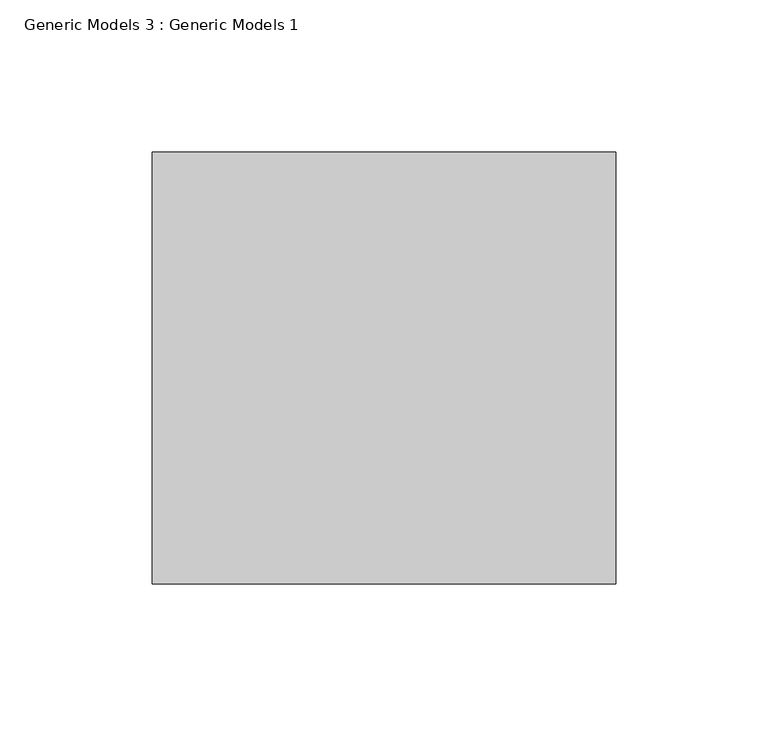
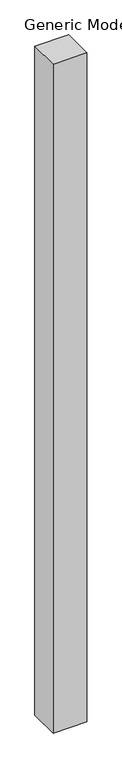
"""IFC4 building model written with IfcOpenShell, lengths in millimetres: proxy geometry, Generic Models 3 : Generic Models 1."""

from ifc_helpers import new_model, si_unit, origin, origin_with_axes, place, context, project, spatial, polyline, outline, extrude, source, transform, mapped, element, save


def generic_models_3_generic_models_1_ed787108(model_context):
    return source(origin(), model_context, "Body", "SweptSolid", [
        extrude(outline(polyline([(-10041.6484471, -5471.7273102), (-9889.2484471, -5471.7273102), (-9889.2484471, -5613.7098142), (-10041.6484471, -5613.7098142), (-10041.6484471, -5471.7273102)])), origin_with_axes(), (0.0, 0.0, 1.0), 3200.4),
    ])


if __name__ == "__main__":
    model = new_model("IFC4")
    model_context = context("Model", 3, world=origin())
    ifc_project = project(units=[si_unit("LENGTHUNIT", "METRE", prefix="MILLI")], contexts=[model_context])
    site = spatial("IfcSite", under=ifc_project)
    building = spatial("IfcBuilding", under=site)
    placement = place(None, origin())
    generic_models_3_generic_models_1_shape = generic_models_3_generic_models_1_ed787108(model_context)
    element("IfcBuildingElementProxy", 1, Name="Generic Models 3 : Generic Models 1", ObjectType="Generic Models 3 : Generic Models 1", at=placement, inside=building, context=model_context, shape_type="MappedRepresentation", body=[
        mapped(generic_models_3_generic_models_1_shape, transform((0.0, 0.0, 0.0), x_axis=(1.0, 0.0, 0.0), y_axis=(0.0, 1.0, 0.0), z_axis=(0.0, 0.0, 1.0))),
    ])
    save(model, "model.ifc")
